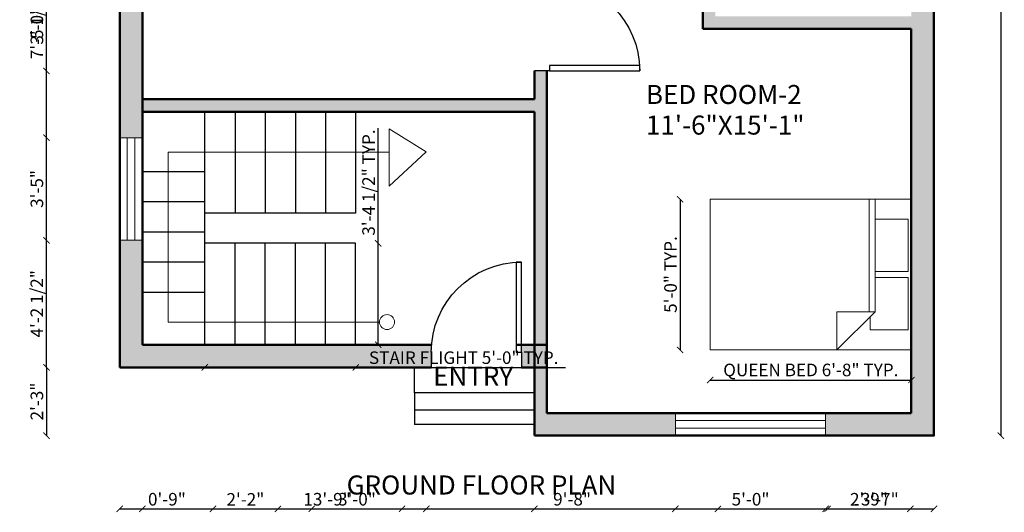
# Model space of a CAD drawing. Units: inches. Extents: x 1799 to 2247, y 1296 to 1881.
# Tile 1 of 4: x 1799 to 2190, y 1296 to 1492. Entities that reach past the tile are written whole.
import ezdxf

# ---------------------------------------------------------------- set-up
doc = ezdxf.new("R2010")
doc.units = ezdxf.units.IN
for name, color, linetype, lineweight in [('A-ANNO-DIMS', 2, 'Continuous', 18), ('A-ANNO-SYMB', 2, 'Continuous', 18), ('A-ANNO-TEXT', 7, 'Continuous', 35), ('A-AREA-IDEN', 7, 'Continuous', 25), ('A-DOOR', 3, 'Continuous', 25), ('A-FLOR-STRS', 7, 'Continuous', 25), ('A-FURN', 8, 'Continuous', 18), ('A-WALL', 7, 'Continuous', 50), ('window', 4, 'Continuous', 18)]:
    doc.layers.add(name, color=color, linetype=linetype, lineweight=lineweight)
doc.layers.add('A-WALL-PATT', color=18, linetype='Continuous', lineweight=13, true_color=0x000000)
doc.styles.get("Standard").update_dxf_attribs({"font": 'arial.ttf'})
doc.dimstyles.new('ISO-25', dxfattribs={"dimtxt": 5, "dimasz": 2.5, "dimexe": 1.25, "dimexo": 0.625, "dimtad": 1, "dimdec": 0, "dimlunit": 4, "dimtxsty": 'Standard', "dimblk": 'ARCHTICK', "dimcen": 2.5, "dimse1": 1, "dimse2": 1, "dimclrd": 1, "dimadec": 0, "dimazin": 0, "dimtfac": 1, "dimtdec": 0, "dimtmove": 0, "dimatfit": 3, "dimfxl": 1, "dimarcsym": 0})

# ---------------------------------------------------------------- blocks, each defined once
blk = doc.blocks.new('Bed - Queen')
for p, q in [((0, -80.00003), (0, 0)), ((0, 0), (59.99999, 0)), ((59.99999, 0), (59.99999, -80.00003)), ((7.99999, -1.2), (28.79998, -1.2)), ((7.99999, -14.4), (7.99999, -1.2)), ((28.79998, -1.2), (28.79998, -14.4)), ((31.19999, -1.2), (51.99999, -1.2)), ((31.19999, -14.4), (31.19999, -1.2)), ((51.99999, -1.2), (51.99999, -16.4)), ((0, -14.4), (44.8, -14.4)), ((59.99999, -29.6), (44.8, -14.4)), ((44.8, -14.4), (44.8, -29.6)), ((44.8, -16.8), (0, -16.8)), ((51.99999, -16.4), (46.79936, -16.4)), ((44.8, -29.6), (59.99999, -29.6)), ((59.99999, -80.00003), (0, -80.00003))]:
    blk.add_line(p, q)
blk = doc.blocks.new('*U12')
for p, q in [((0, 0), (0, -5)), ((30, 0), (30, -5))]:
    blk.add_line(p, q)
blk.add_lwpolyline([(0, 0), (0, 30), (1.75, 30), (1.75, 0)], close=True)
blk.add_arc((0, 0), 30, 0, 90)
blk = doc.blocks.new('_ArchTick')
at = {"color": 0, "linetype": 'ByBlock', "const_width": 0.15}
blk.add_lwpolyline([(-0.5, -0.5), (0.5, 0.5)], dxfattribs=at)
blk = doc.blocks.new('*D14')
at = {"layer": 'A-ANNO-DIMS', "color": 0, "lineweight": -2, "transparency": 16777216}
blk.add_line((2189.08, 1830.32), (2189.08, 1326.32), dxfattribs=at)
at = {"layer": 'Defpoints', "color": 0, "transparency": 16777216}
for p in [(2162.46, 1830.32), (2162.46, 1326.32), (2189.08, 1326.32)]:
    blk.add_point(p, dxfattribs=at)
at = {"layer": 'A-ANNO-DIMS', "color": 0, "lineweight": -2, "transparency": 16777216, "xscale": 2.5, "yscale": 2.5, "zscale": 2.5}
for p, rotation in [((2189.08, 1830.32), 90), ((2189.08, 1326.32), 270)]:
    blk.add_blockref('_ArchTick', p, dxfattribs=dict(at, rotation=rotation))
at = {"layer": 'A-ANNO-DIMS', "color": 0, "transparency": 16777216, "insert": (2185.95, 1578.32), "char_height": 5, "attachment_point": 5, "rotation": 90}
blk.add_mtext("42'", dxfattribs=at)
blk = doc.blocks.new('STAIR-FLIGHT-5-TREAD')
for p, q in [((60, 40.41), (0, 40.41)), ((12, 0), (12, 40.41)), ((24, 0), (24, 40.41)), ((36, 0), (36, 40.41)), ((48, 0), (48, 40.41)), ((60, 0), (60, 40.41))]:
    blk.add_line(p, q)
blk = doc.blocks.new('*D16')
at = {"layer": 'A-ANNO-DIMS', "color": 1, "lineweight": -2, "transparency": 16777216}
blk.add_line((2073.46, 1348.47), (2153.46, 1348.47), dxfattribs=at)
at = {"layer": 'Defpoints', "color": 0, "transparency": 16777216}
for p in [(2073.46, 1360.47), (2153.46, 1360.47), (2153.46, 1348.47)]:
    blk.add_point(p, dxfattribs=at)
at = {"layer": 'A-ANNO-DIMS', "color": 1, "lineweight": -2, "transparency": 16777216, "xscale": 2.5, "yscale": 2.5, "zscale": 2.5, "rotation": 180}
blk.add_blockref('_ArchTick', (2073.46, 1348.47), dxfattribs=at)
at = {"layer": 'A-ANNO-DIMS', "color": 1, "lineweight": -2, "transparency": 16777216, "xscale": 2.5, "yscale": 2.5, "zscale": 2.5}
blk.add_blockref('_ArchTick', (2153.46, 1348.47), dxfattribs=at)
at = {"layer": 'A-ANNO-DIMS', "color": 0, "transparency": 16777216, "insert": (2113.46, 1351.83), "char_height": 5, "attachment_point": 5}
blk.add_mtext('QUEEN BED 6\'-8" TYP.', dxfattribs=at)
blk = doc.blocks.new('*D17')
at = {"layer": 'A-ANNO-DIMS', "color": 1, "lineweight": -2, "transparency": 16777216}
blk.add_line((2061.46, 1420.47), (2061.46, 1360.47), dxfattribs=at)
at = {"layer": 'Defpoints', "color": 0, "transparency": 16777216}
for p in [(2073.46, 1420.47), (2061.46, 1360.47), (2073.46, 1360.47)]:
    blk.add_point(p, dxfattribs=at)
at = {"layer": 'A-ANNO-DIMS', "color": 1, "lineweight": -2, "transparency": 16777216, "xscale": 2.5, "yscale": 2.5, "zscale": 2.5}
for p, rotation in [((2061.46, 1420.47), 90), ((2061.46, 1360.47), 270)]:
    blk.add_blockref('_ArchTick', p, dxfattribs=dict(at, rotation=rotation))
at = {"layer": 'A-ANNO-DIMS', "color": 0, "transparency": 16777216, "insert": (2058.28, 1390.47), "char_height": 5, "attachment_point": 5, "rotation": 90}
blk.add_mtext('5\'-0" TYP.', dxfattribs=at)
blk = doc.blocks.new('*D20')
at = {"layer": 'A-ANNO-DIMS', "color": 1, "lineweight": -2, "transparency": 16777216}
for p, q in [((1872.34, 1353.51), (1932.34, 1353.51)), ((1932.34, 1353.51), (2015.83, 1353.51))]:
    blk.add_line(p, q, dxfattribs=at)
at = {"layer": 'Defpoints', "color": 0, "transparency": 16777216}
for p in [(1872.34, 1362.51), (1932.34, 1362.51), (1932.34, 1353.51)]:
    blk.add_point(p, dxfattribs=at)
at = {"layer": 'A-ANNO-DIMS', "color": 1, "lineweight": -2, "transparency": 16777216, "xscale": 2.5, "yscale": 2.5, "zscale": 2.5, "rotation": 180}
blk.add_blockref('_ArchTick', (1872.34, 1353.51), dxfattribs=at)
at = {"layer": 'A-ANNO-DIMS', "color": 1, "lineweight": -2, "transparency": 16777216, "xscale": 2.5, "yscale": 2.5, "zscale": 2.5}
blk.add_blockref('_ArchTick', (1932.34, 1353.51), dxfattribs=at)
at = {"layer": 'A-ANNO-DIMS', "color": 0, "transparency": 16777216, "insert": (1975.33, 1356.72), "char_height": 5, "attachment_point": 5}
blk.add_mtext('STAIR FLIGHT 5\'-0" TYP.', dxfattribs=at)
blk = doc.blocks.new('*D21')
at = {"layer": 'A-ANNO-DIMS', "color": 1, "lineweight": -2, "transparency": 16777216}
for p, q in [((1941.34, 1402.91), (1941.34, 1448.79)), ((1941.34, 1362.51), (1941.34, 1402.91))]:
    blk.add_line(p, q, dxfattribs=at)
at = {"layer": 'Defpoints', "color": 0, "transparency": 16777216}
for p in [(1932.34, 1402.91), (1941.34, 1402.91), (1932.34, 1362.51)]:
    blk.add_point(p, dxfattribs=at)
at = {"layer": 'A-ANNO-DIMS', "color": 1, "lineweight": -2, "transparency": 16777216, "xscale": 2.5, "yscale": 2.5, "zscale": 2.5}
for p, rotation in [((1941.34, 1402.91), 90), ((1941.34, 1362.51), 270)]:
    blk.add_blockref('_ArchTick', p, dxfattribs=dict(at, rotation=rotation))
at = {"layer": 'A-ANNO-DIMS', "color": 0, "transparency": 16777216, "insert": (1938.13, 1427.1), "char_height": 5, "attachment_point": 5, "rotation": 90}
blk.add_mtext('3\'-4 1/2" TYP.', dxfattribs=at)
blk = doc.blocks.new('*D32')
at = {"layer": 'A-ANNO-DIMS', "color": 1, "lineweight": -2, "transparency": 16777216}
blk.add_line((1838.46, 1297.17), (2003.46, 1297.17), dxfattribs=at)
at = {"layer": 'Defpoints', "color": 0, "transparency": 16777216}
for p in [(1838.46, 1353.51), (2003.46, 1326.32), (2003.46, 1297.17)]:
    blk.add_point(p, dxfattribs=at)
at = {"layer": 'A-ANNO-DIMS', "color": 1, "lineweight": -2, "transparency": 16777216, "xscale": 2.5, "yscale": 2.5, "zscale": 2.5, "rotation": 180}
blk.add_blockref('_ArchTick', (1838.46, 1297.17), dxfattribs=at)
at = {"layer": 'A-ANNO-DIMS', "color": 1, "lineweight": -2, "transparency": 16777216, "xscale": 2.5, "yscale": 2.5, "zscale": 2.5}
blk.add_blockref('_ArchTick', (2003.46, 1297.17), dxfattribs=at)
at = {"layer": 'A-ANNO-DIMS', "color": 0, "transparency": 16777216, "insert": (1920.96, 1300.35), "char_height": 5, "attachment_point": 5}
blk.add_mtext('13\'-9"', dxfattribs=at)
blk = doc.blocks.new('*D33')
at = {"layer": 'A-ANNO-DIMS', "color": 1, "lineweight": -2, "transparency": 16777216}
blk.add_line((1809.31, 1353.51), (1809.31, 1326.32), dxfattribs=at)
at = {"layer": 'Defpoints', "color": 0, "transparency": 16777216}
for p in [(1838.46, 1353.51), (1809.31, 1326.32), (2003.46, 1326.32)]:
    blk.add_point(p, dxfattribs=at)
at = {"layer": 'A-ANNO-DIMS', "color": 1, "lineweight": -2, "transparency": 16777216, "xscale": 2.5, "yscale": 2.5, "zscale": 2.5}
for p, rotation in [((1809.31, 1353.51), 90), ((1809.31, 1326.32), 270)]:
    blk.add_blockref('_ArchTick', p, dxfattribs=dict(at, rotation=rotation))
at = {"layer": 'A-ANNO-DIMS', "color": 0, "transparency": 16777216, "insert": (1806.13, 1339.91), "char_height": 5, "attachment_point": 5, "rotation": 90}
blk.add_mtext('2\'-3"', dxfattribs=at)
blk = doc.blocks.new('*D35')
at = {"layer": 'A-ANNO-DIMS', "color": 1, "lineweight": -2, "transparency": 16777216}
blk.add_line((1960.46, 1297.17), (2076.46, 1297.17), dxfattribs=at)
at = {"layer": 'Defpoints', "color": 0, "transparency": 16777216}
for p in [(1960.46, 1821.32), (2076.46, 1821.32), (2076.46, 1297.17)]:
    blk.add_point(p, dxfattribs=at)
at = {"layer": 'A-ANNO-DIMS', "color": 1, "lineweight": -2, "transparency": 16777216, "xscale": 2.5, "yscale": 2.5, "zscale": 2.5, "rotation": 180}
blk.add_blockref('_ArchTick', (1960.46, 1297.17), dxfattribs=at)
at = {"layer": 'A-ANNO-DIMS', "color": 1, "lineweight": -2, "transparency": 16777216, "xscale": 2.5, "yscale": 2.5, "zscale": 2.5}
blk.add_blockref('_ArchTick', (2076.46, 1297.17), dxfattribs=at)
at = {"layer": 'A-ANNO-DIMS', "color": 0, "transparency": 16777216, "insert": (2018.46, 1300.35), "char_height": 5, "attachment_point": 5}
blk.add_mtext('9\'-8"', dxfattribs=at)
blk = doc.blocks.new('*D37')
at = {"layer": 'A-ANNO-DIMS', "color": 1, "lineweight": -2, "transparency": 16777216}
blk.add_line((2119.37, 1297.17), (2162.46, 1297.17), dxfattribs=at)
at = {"layer": 'Defpoints', "color": 0, "transparency": 16777216}
for p in [(2119.37, 1326.32), (2162.46, 1326.32), (2162.46, 1297.17)]:
    blk.add_point(p, dxfattribs=at)
at = {"layer": 'A-ANNO-DIMS', "color": 1, "lineweight": -2, "transparency": 16777216, "xscale": 2.5, "yscale": 2.5, "zscale": 2.5, "rotation": 180}
blk.add_blockref('_ArchTick', (2119.37, 1297.17), dxfattribs=at)
at = {"layer": 'A-ANNO-DIMS', "color": 1, "lineweight": -2, "transparency": 16777216, "xscale": 2.5, "yscale": 2.5, "zscale": 2.5}
blk.add_blockref('_ArchTick', (2162.46, 1297.17), dxfattribs=at)
at = {"layer": 'A-ANNO-DIMS', "color": 0, "transparency": 16777216, "insert": (2140.92, 1300.35), "char_height": 5, "attachment_point": 5}
blk.add_mtext('3\'-7"', dxfattribs=at)
blk = doc.blocks.new('*D38')
at = {"layer": 'A-ANNO-DIMS', "color": 1, "lineweight": -2, "transparency": 16777216}
blk.add_line((2059.58, 1297.17), (2119.37, 1297.17), dxfattribs=at)
at = {"layer": 'Defpoints', "color": 0, "transparency": 16777216}
for p in [(2059.58, 1326.32), (2119.37, 1326.32), (2119.37, 1297.17)]:
    blk.add_point(p, dxfattribs=at)
at = {"layer": 'A-ANNO-DIMS', "color": 1, "lineweight": -2, "transparency": 16777216, "xscale": 2.5, "yscale": 2.5, "zscale": 2.5, "rotation": 180}
blk.add_blockref('_ArchTick', (2059.58, 1297.17), dxfattribs=at)
at = {"layer": 'A-ANNO-DIMS', "color": 1, "lineweight": -2, "transparency": 16777216, "xscale": 2.5, "yscale": 2.5, "zscale": 2.5}
blk.add_blockref('_ArchTick', (2119.37, 1297.17), dxfattribs=at)
at = {"layer": 'A-ANNO-DIMS', "color": 0, "transparency": 16777216, "insert": (2089.48, 1300.35), "char_height": 5, "attachment_point": 5}
blk.add_mtext('5\'-0"', dxfattribs=at)
blk = doc.blocks.new('*D47')
at = {"layer": 'A-ANNO-DIMS', "color": 1, "lineweight": -2, "transparency": 16777216}
blk.add_line((1914.89, 1297.17), (1950.83, 1297.17), dxfattribs=at)
at = {"layer": 'Defpoints', "color": 0, "transparency": 16777216}
for p in [(1914.89, 1701.32), (1950.83, 1701.32), (1950.83, 1297.17)]:
    blk.add_point(p, dxfattribs=at)
at = {"layer": 'A-ANNO-DIMS', "color": 1, "lineweight": -2, "transparency": 16777216, "xscale": 2.5, "yscale": 2.5, "zscale": 2.5, "rotation": 180}
blk.add_blockref('_ArchTick', (1914.89, 1297.17), dxfattribs=at)
at = {"layer": 'A-ANNO-DIMS', "color": 1, "lineweight": -2, "transparency": 16777216, "xscale": 2.5, "yscale": 2.5, "zscale": 2.5}
blk.add_blockref('_ArchTick', (1950.83, 1297.17), dxfattribs=at)
at = {"layer": 'A-ANNO-DIMS', "color": 0, "transparency": 16777216, "insert": (1932.86, 1300.35), "char_height": 5, "attachment_point": 5}
blk.add_mtext('3\'-0"', dxfattribs=at)
blk = doc.blocks.new('*D48')
at = {"layer": 'A-ANNO-DIMS', "color": 1, "lineweight": -2, "transparency": 16777216}
blk.add_line((1962.42, 1859.47), (1998.36, 1859.47), dxfattribs=at)
at = {"layer": 'Defpoints', "color": 0, "transparency": 16777216}
for p in [(1998.36, 1859.47), (1962.42, 1353.51), (1998.36, 1353.51)]:
    blk.add_point(p, dxfattribs=at)
at = {"layer": 'A-ANNO-DIMS', "color": 1, "lineweight": -2, "transparency": 16777216, "xscale": 2.5, "yscale": 2.5, "zscale": 2.5, "rotation": 180}
blk.add_blockref('_ArchTick', (1962.42, 1859.47), dxfattribs=at)
at = {"layer": 'A-ANNO-DIMS', "color": 1, "lineweight": -2, "transparency": 16777216, "xscale": 2.5, "yscale": 2.5, "zscale": 2.5}
blk.add_blockref('_ArchTick', (1998.36, 1859.47), dxfattribs=at)
at = {"layer": 'A-ANNO-DIMS', "color": 0, "transparency": 16777216, "insert": (1980.39, 1862.65), "char_height": 5, "attachment_point": 5}
blk.add_mtext('3\'-0"', dxfattribs=at)
blk = doc.blocks.new('*D50')
at = {"layer": 'A-ANNO-DIMS', "color": 1, "lineweight": -2, "transparency": 16777216}
blk.add_line((1809.31, 1444.97), (1809.31, 1534.31), dxfattribs=at)
at = {"layer": 'Defpoints', "color": 0, "transparency": 16777216}
for p in [(1809.31, 1534.31), (1838.46, 1534.31), (1838.46, 1444.97)]:
    blk.add_point(p, dxfattribs=at)
at = {"layer": 'A-ANNO-DIMS', "color": 1, "lineweight": -2, "transparency": 16777216, "xscale": 2.5, "yscale": 2.5, "zscale": 2.5}
for p, rotation in [((1809.31, 1534.31), 90), ((1809.31, 1444.97), 270)]:
    blk.add_blockref('_ArchTick', p, dxfattribs=dict(at, rotation=rotation))
at = {"layer": 'A-ANNO-DIMS', "color": 0, "transparency": 16777216, "insert": (1806.1, 1489.64), "char_height": 5, "attachment_point": 5, "rotation": 90}
blk.add_mtext('7\'-5 1/2"', dxfattribs=at)
blk = doc.blocks.new('*D51')
at = {"layer": 'A-ANNO-DIMS', "color": 1, "lineweight": -2, "transparency": 16777216}
blk.add_line((1809.31, 1404.13), (1809.31, 1444.97), dxfattribs=at)
at = {"layer": 'Defpoints', "color": 0, "transparency": 16777216}
for p in [(1809.31, 1444.97), (1838.46, 1444.97), (1838.46, 1404.13)]:
    blk.add_point(p, dxfattribs=at)
at = {"layer": 'A-ANNO-DIMS', "color": 1, "lineweight": -2, "transparency": 16777216, "xscale": 2.5, "yscale": 2.5, "zscale": 2.5}
for p, rotation in [((1809.31, 1444.97), 90), ((1809.31, 1404.13), 270)]:
    blk.add_blockref('_ArchTick', p, dxfattribs=dict(at, rotation=rotation))
at = {"layer": 'A-ANNO-DIMS', "color": 0, "transparency": 16777216, "insert": (1806.13, 1424.55), "char_height": 5, "attachment_point": 5, "rotation": 90}
blk.add_mtext('3\'-5"', dxfattribs=at)
blk = doc.blocks.new('*D52')
at = {"layer": 'A-ANNO-DIMS', "color": 1, "lineweight": -2, "transparency": 16777216}
blk.add_line((1809.31, 1353.51), (1809.31, 1404.13), dxfattribs=at)
at = {"layer": 'Defpoints', "color": 0, "transparency": 16777216}
for p in [(1809.31, 1404.13), (1838.46, 1404.13), (1838.46, 1353.51)]:
    blk.add_point(p, dxfattribs=at)
at = {"layer": 'A-ANNO-DIMS', "color": 1, "lineweight": -2, "transparency": 16777216, "xscale": 2.5, "yscale": 2.5, "zscale": 2.5}
for p, rotation in [((1809.31, 1404.13), 90), ((1809.31, 1353.51), 270)]:
    blk.add_blockref('_ArchTick', p, dxfattribs=dict(at, rotation=rotation))
at = {"layer": 'A-ANNO-DIMS', "color": 0, "transparency": 16777216, "insert": (1806.1, 1378.82), "char_height": 5, "attachment_point": 5, "rotation": 90}
blk.add_mtext('4\'-2 1/2"', dxfattribs=at)
blk = doc.blocks.new('*D57')
at = {"layer": 'A-ANNO-DIMS', "color": 1, "lineweight": -2, "transparency": 16777216}
blk.add_line((1875.53, 1297.17), (1901.39, 1297.17), dxfattribs=at)
at = {"layer": 'Defpoints', "color": 0, "transparency": 16777216}
for p in [(1901.39, 1801.76), (1875.53, 1797.03), (1901.39, 1297.17)]:
    blk.add_point(p, dxfattribs=at)
at = {"layer": 'A-ANNO-DIMS', "color": 1, "lineweight": -2, "transparency": 16777216, "xscale": 2.5, "yscale": 2.5, "zscale": 2.5, "rotation": 180}
blk.add_blockref('_ArchTick', (1875.53, 1297.17), dxfattribs=at)
at = {"layer": 'A-ANNO-DIMS', "color": 1, "lineweight": -2, "transparency": 16777216, "xscale": 2.5, "yscale": 2.5, "zscale": 2.5}
blk.add_blockref('_ArchTick', (1901.39, 1297.17), dxfattribs=at)
at = {"layer": 'A-ANNO-DIMS', "color": 0, "transparency": 16777216, "insert": (1888.46, 1300.3), "char_height": 5, "attachment_point": 5}
blk.add_mtext('2\'-2"', dxfattribs=at)
blk = doc.blocks.new('*D60')
at = {"layer": 'A-ANNO-DIMS', "color": 1, "lineweight": -2, "transparency": 16777216}
blk.add_line((1809.31, 1471.58), (1809.31, 1507.52), dxfattribs=at)
at = {"layer": 'Defpoints', "color": 0, "transparency": 16777216}
for p in [(1809.31, 1507.52), (2003.46, 1507.52), (2003.46, 1471.58)]:
    blk.add_point(p, dxfattribs=at)
at = {"layer": 'A-ANNO-DIMS', "color": 1, "lineweight": -2, "transparency": 16777216, "xscale": 2.5, "yscale": 2.5, "zscale": 2.5}
for p, rotation in [((1809.31, 1507.52), 90), ((1809.31, 1471.58), 270)]:
    blk.add_blockref('_ArchTick', p, dxfattribs=dict(at, rotation=rotation))
at = {"layer": 'A-ANNO-DIMS', "color": 0, "transparency": 16777216, "insert": (1806.13, 1489.55), "char_height": 5, "attachment_point": 5, "rotation": 90}
blk.add_mtext('3\'-0"', dxfattribs=at)
blk = doc.blocks.new('*D61')
at = {"layer": 'A-ANNO-DIMS', "color": 1, "lineweight": -2, "transparency": 16777216}
for p, q in [((1838.46, 1297.17), (1847.46, 1297.17)), ((1847.46, 1297.17), (1864.5, 1297.17))]:
    blk.add_line(p, q, dxfattribs=at)
at = {"layer": 'Defpoints', "color": 0, "transparency": 16777216}
for p in [(1838.46, 1830.32), (1847.46, 1821.32), (1847.46, 1297.17)]:
    blk.add_point(p, dxfattribs=at)
at = {"layer": 'A-ANNO-DIMS', "color": 1, "lineweight": -2, "transparency": 16777216, "xscale": 2.5, "yscale": 2.5, "zscale": 2.5, "rotation": 180}
blk.add_blockref('_ArchTick', (1838.46, 1297.17), dxfattribs=at)
at = {"layer": 'A-ANNO-DIMS', "color": 1, "lineweight": -2, "transparency": 16777216, "xscale": 2.5, "yscale": 2.5, "zscale": 2.5}
blk.add_blockref('_ArchTick', (1847.46, 1297.17), dxfattribs=at)
at = {"layer": 'A-ANNO-DIMS', "color": 0, "transparency": 16777216, "insert": (1857.23, 1300.35), "char_height": 5, "attachment_point": 5}
blk.add_mtext('0\'-9"', dxfattribs=at)
blk = doc.blocks.new('*D66')
at = {"layer": 'A-ANNO-DIMS', "color": 1, "lineweight": -2, "transparency": 16777216}
blk.add_line((2120.1, 1297.17), (2153.1, 1297.17), dxfattribs=at)
at = {"layer": 'Defpoints', "color": 0, "transparency": 16777216}
for p in [(2120.1, 1525.25), (2153.1, 1514.75), (2153.1, 1297.17)]:
    blk.add_point(p, dxfattribs=at)
at = {"layer": 'A-ANNO-DIMS', "color": 1, "lineweight": -2, "transparency": 16777216, "xscale": 2.5, "yscale": 2.5, "zscale": 2.5, "rotation": 180}
blk.add_blockref('_ArchTick', (2120.1, 1297.17), dxfattribs=at)
at = {"layer": 'A-ANNO-DIMS', "color": 1, "lineweight": -2, "transparency": 16777216, "xscale": 2.5, "yscale": 2.5, "zscale": 2.5}
blk.add_blockref('_ArchTick', (2153.1, 1297.17), dxfattribs=at)
at = {"layer": 'A-ANNO-DIMS', "color": 0, "transparency": 16777216, "insert": (2136.6, 1300.35), "char_height": 5, "attachment_point": 5}
blk.add_mtext('2\'-9"', dxfattribs=at)

msp = doc.modelspace()

# ---------------------------------------------------------------- hatches: boundary and pattern name
at = {"layer": 'A-WALL-PATT'}
h = msp.add_hatch(color=256, dxfattribs=at)
h.dxf.hatch_style = 1
h.paths.add_polyline_path([(1847.46, 1821.32), (1883.11, 1821.32), (1883.11, 1830.32), (1838.46, 1830.32), (1838.46, 1618.8), (1847.46, 1618.8)])
h.paths.add_polyline_path([(1847.46, 1534.31), (1838.46, 1534.31), (1838.46, 1444.97), (1847.46, 1444.97)])
h.paths.add_polyline_path([(1847.46, 1404.13), (1838.46, 1404.13), (1838.46, 1353.51), (1847.46, 1353.51), (1962.42, 1353.51), (1962.42, 1359.5, -0.020971), (1962.55, 1362.51), (1847.46, 1362.51)])
h.paths.add_polyline_path([(2162.46, 1509.73), (2153.46, 1509.73), (2153.46, 1493.32), (2075.46, 1493.32), (2075.46, 1496.56), (2075.02, 1496.56), (2070.46, 1496.56), (2070.46, 1488.32), (2153.46, 1488.32), (2153.46, 1335.32), (2119.37, 1335.32), (2119.37, 1326.32), (2162.46, 1326.32)])
h.paths.add_polyline_path([(2059.58, 1335.32), (2008.46, 1335.32), (2008.46, 1353.51), (2003.46, 1353.51), (2003.46, 1335.32), (2003.46, 1326.32), (2059.58, 1326.32)])
h.paths.add_polyline_path([(2008.46, 1471.58), (2003.46, 1471.58), (2003.46, 1460.32), (1847.46, 1460.32), (1847.46, 1455.32), (2003.46, 1455.32), (2003.46, 1362.51), (2008.46, 1362.51)])
h.paths.add_polyline_path([(2008.46, 1362.51), (2003.46, 1362.51), (2003.46, 1353.51), (2008.46, 1353.51)])
h.paths.add_polyline_path([(2003.46, 1362.51), (1998.36, 1362.51), (1998.36, 1359.5), (1998.36, 1353.51), (2003.46, 1353.51)])
h.paths.add_polyline_path([(1989.49, 1830.32), (1953.2, 1830.32), (1953.2, 1821.32), (1955.46, 1821.32), (1955.46, 1701.32), (1950.83, 1701.32), (1950.83, 1696.32), (1960.46, 1696.32), (1960.46, 1821.32), (1989.49, 1821.32)])
h.paths.add_polyline_path([(2162.46, 1606.83), (2153.46, 1606.83), (2153.46, 1541.93), (2162.46, 1541.93)])
h.paths.add_polyline_path([(2162.46, 1746.71), (2153.46, 1746.71), (2153.46, 1701.32), (2081.46, 1701.32), (2081.46, 1707.91), (2081.05, 1707.91), (2076.46, 1707.91), (2076.46, 1701.32), (2003.46, 1701.32), (2003.46, 1604.81), (2008.46, 1604.81), (2008.46, 1696.32), (2153.46, 1696.32), (2153.46, 1656.83), (2162.46, 1656.83)])
h.paths.add_polyline_path([(2162.46, 1830.32), (2050.89, 1830.32), (2050.89, 1821.32), (2076.46, 1821.32), (2076.46, 1735.44), (2081.05, 1735.44, -0.003736), (2081.46, 1735.44), (2081.46, 1821.32), (2153.46, 1821.32), (2153.46, 1778.8), (2162.46, 1778.8)])
h.paths.add_polyline_path([(1961.29, 1344.27), (2000.99, 1344.27), (2000.99, 1355.65), (1961.29, 1355.65)], flags=9)
h.paths.add_polyline_path([(1882.83, 1491.06), (1947.74, 1491.06), (1947.74, 1502.69), (1882.83, 1502.69)], flags=9)
h.paths.add_polyline_path([(1882.8, 1503.23), (1950.9, 1503.23), (1950.9, 1514.99), (1882.8, 1514.99)], flags=9)
h.paths.add_polyline_path([(2045.91, 1444.14), (2110.82, 1444.14), (2110.82, 1455.75), (2045.91, 1455.75)], flags=9)
h.paths.add_polyline_path([(2045.88, 1456.29), (2116.91, 1456.29), (2116.91, 1468.06), (2045.88, 1468.06)], flags=9)
h.paths.add_polyline_path([(2084.43, 1526.38), (2124.38, 1526.38), (2124.38, 1537.99), (2084.43, 1537.99)], flags=9)
h.paths.add_polyline_path([(2084.4, 1538.53), (2125.41, 1538.53), (2125.41, 1550.3), (2084.4, 1550.3)], flags=9)
h.paths.add_polyline_path([(2013.59, 1530.05), (2066.72, 1530.05), (2066.72, 1541.67), (2013.59, 1541.67)], flags=9)
h.paths.add_polyline_path([(2013.56, 1542.21), (2053.98, 1542.21), (2053.98, 1553.97), (2013.56, 1553.97)], flags=9)
h.paths.add_polyline_path([(2054.17, 1583.99), (2119.08, 1583.99), (2119.08, 1595.62), (2054.17, 1595.62)], flags=9)
h.paths.add_polyline_path([(2054.14, 1596.16), (2125.17, 1596.16), (2125.17, 1607.93), (2054.14, 1607.93)], flags=9)
h.paths.add_polyline_path([(2091.32, 1783.78), (2144.45, 1783.78), (2144.45, 1795.39), (2091.32, 1795.39)], flags=25)
h.paths.add_polyline_path([(2091.3, 1795.93), (2142.9, 1795.93), (2142.9, 1807.7), (2091.3, 1807.7)], flags=25)
h.paths.add_polyline_path([(1985.13, 1779.5), (2017.8, 1779.5), (2017.8, 1790.88), (1985.13, 1790.88)], flags=9)
h.paths.add_polyline_path([(1985.08, 1791.49), (2020.79, 1791.49), (2020.79, 1803.25), (1985.08, 1803.25)], flags=9)
h.paths.add_polyline_path([(1879.15, 1761.55), (1938.17, 1761.55), (1938.17, 1773.17), (1879.15, 1773.17)], flags=9)
h.paths.add_polyline_path([(1879.13, 1773.71), (1929.55, 1773.71), (1929.55, 1785.47), (1879.13, 1785.47)], flags=9)

# ---------------------------------------------------------------- linework, layer by layer
at = {"layer": 'A-ANNO-SYMB'}
for p, q in [((1945.62, 1439.15), (1945.62, 1448.48)), ((1945.62, 1448.48), (1960.37, 1439.27)), ((1857.67, 1371.55), (1857.67, 1439.15)), ((1857.67, 1439.15), (1945.62, 1439.15)), ((1960.37, 1439.27), (1945.62, 1425.67)), ((1945.62, 1425.67), (1945.62, 1439.15)), ((1941.83, 1371.55), (1857.67, 1371.55))]:
    msp.add_line(p, q, dxfattribs=at)
msp.add_circle((1944.82, 1371.55), 2.99, dxfattribs=at)
at = {"layer": 'A-FLOR-STRS'}
for p, q in [((1872.34, 1362.51), (1872.34, 1455.32)), ((1872.34, 1431.38), (1847.46, 1431.38)), ((1872.34, 1419.38), (1847.46, 1419.38)), ((1872.34, 1407.38), (1847.46, 1407.38)), ((1872.34, 1395.38), (1847.46, 1395.38)), ((1872.34, 1383.38), (1847.46, 1383.38)), ((1955.8, 1343.4), (1955.8, 1353.51)), ((2003.46, 1343.4), (1955.8, 1343.4)), ((1955.8, 1343.4), (1955.8, 1330.82)), ((2003.46, 1336.5), (1955.8, 1336.5)), ((2003.46, 1330.82), (1955.8, 1330.82))]:
    msp.add_line(p, q, dxfattribs=at)
at = {"layer": 'A-WALL'}
for p, q in [((1847.46, 1362.51), (1847.46, 1821.32)), ((2070.46, 1496.56), (2070.46, 1488.32)), ((2070.46, 1488.32), (2153.46, 1488.32)), ((2153.46, 1488.32), (2153.46, 1335.32)), ((2003.46, 1460.32), (2003.46, 1471.58)), ((2008.46, 1335.32), (2008.46, 1471.58)), ((1847.46, 1460.32), (2003.46, 1460.32)), ((1847.46, 1455.32), (2003.46, 1455.32)), ((2003.46, 1335.32), (2003.46, 1455.32)), ((1847.46, 1362.51), (1962.55, 1362.51)), ((1996.26, 1362.51), (2008.46, 1362.51)), ((1847.46, 1353.51), (1838.46, 1353.51)), ((1847.46, 1353.51), (1962.42, 1353.51)), ((1998.36, 1353.51), (2008.46, 1353.51)), ((2003.46, 1335.32), (2003.46, 1326.32)), ((2153.46, 1335.32), (2008.46, 1335.32))]:
    msp.add_line(p, q, dxfattribs=at)
msp.add_lwpolyline([(1838.46, 1353.51), (1838.46, 1830.32), (2162.46, 1830.32), (2162.46, 1326.32), (2003.46, 1326.32)], dxfattribs=at)
at = {"layer": 'window'}
for p, q in [((1847.46, 1444.97), (1838.46, 1444.97)), ((1838.46, 1444.97), (1838.46, 1404.13)), ((1841.46, 1444.97), (1841.46, 1404.13)), ((1844.46, 1444.97), (1844.46, 1404.13)), ((1847.46, 1404.13), (1847.46, 1444.97)), ((1838.46, 1404.13), (1847.46, 1404.13)), ((2059.58, 1335.32), (2059.58, 1326.32)), ((2119.37, 1335.32), (2059.58, 1335.32)), ((2059.58, 1332.32), (2119.37, 1332.32)), ((2119.37, 1326.32), (2119.37, 1335.32)), ((2059.58, 1329.32), (2119.37, 1329.32)), ((2059.58, 1326.32), (2119.37, 1326.32))]:
    msp.add_line(p, q, dxfattribs=at)

# ---------------------------------------------------------------- block references
at = {"layer": 'A-DOOR', "xscale": -1.197883670562129, "yscale": 1.197883670562129, "zscale": 1.197883670562129, "rotation": 270}
msp.add_blockref('*U12', (2009.45, 1471.58), dxfattribs=at)
at = {"layer": 'A-DOOR', "xscale": -1.197883670562129, "yscale": 1.197883670562129, "zscale": 1.197883670562129}
msp.add_blockref('*U12', (1998.36, 1359.5), dxfattribs=at)
at = {"layer": 'A-FLOR-STRS', "extrusion": (0, 0, -1), "zscale": -1, "rotation": 180}
msp.add_blockref('STAIR-FLIGHT-5-TREAD', (-1872.34, 1455.32), dxfattribs=at)
at = {"layer": 'A-FLOR-STRS'}
msp.add_blockref('STAIR-FLIGHT-5-TREAD', (1872.34, 1362.51), dxfattribs=at)
at = {"layer": 'A-FURN', "rotation": 270}
msp.add_blockref('Bed - Queen', (2153.46, 1420.47), dxfattribs=at)

# ---------------------------------------------------------------- texts
at = {"layer": 'A-ANNO-TEXT'}
msp.add_text('GROUND FLOOR PLAN', height=7.5834, dxfattribs=at).set_placement((1928.74, 1302.88))
at = {"layer": 'A-AREA-IDEN'}
for s, height, p in [('BED ROOM-2', 7.583, (2047.85, 1458.38)), ('11\'-6"X15\'-1"', 7.5834, (2047.85, 1446.2)), ('ENTRY', 7.583, (1963.19, 1346.17))]:
    msp.add_text(s, height=height, dxfattribs=at).set_placement(p)

# ---------------------------------------------------------------- dimensions: what is measured, and where the dimension line sits
at = {"layer": 'A-ANNO-DIMS'}
for base, p1, p2, picture, middle in [((1998.36, 1859.47), (1962.42, 1353.51), (1998.36, 1353.51), '*D48', (1980.39, 1862.65)), ((1847.46, 1297.17), (1838.46, 1830.32), (1847.46, 1821.32), '*D61', (1857.23, 1300.35)), ((2076.46, 1297.17), (1960.46, 1821.32), (2076.46, 1821.32), '*D35', (2018.46, 1300.35)), ((1901.39, 1297.17), (1875.53, 1797.03), (1901.39, 1801.76), '*D57', (1888.46, 1300.3)), ((1950.83, 1297.17), (1914.89, 1701.32), (1950.83, 1701.32), '*D47', (1932.86, 1300.35)), ((2153.1, 1297.17), (2120.1, 1525.25), (2153.1, 1514.75), '*D66', (2136.6, 1300.35)), ((2003.46, 1297.17), (1838.46, 1353.51), (2003.46, 1326.32), '*D32', (1920.96, 1300.35)), ((2119.37, 1297.17), (2059.58, 1326.32), (2119.37, 1326.32), '*D38', (2089.48, 1300.35)), ((2162.46, 1297.17), (2119.37, 1326.32), (2162.46, 1326.32), '*D37', (2140.92, 1300.35))]:
    dim = msp.add_linear_dim(base=base, p1=p1, p2=p2, dimstyle='ISO-25', override={"dimdec": 1, "dimlfac": 1, "dimrnd": 0, "dimzin": 1, "dimdsep": 46, "dimlunit": 4, "dimfrac": 2}, dxfattribs=at)
    dim.commit()
    dim.dimension.update_dxf_attribs({"geometry": picture, "text_midpoint": middle})
for base, p1, p2, override, picture, middle in [((2189.08, 1326.32), (2162.46, 1830.32), (2162.46, 1326.32), {"dimclrd": 0, "dimclre": 0, "dimclrt": 0}, '*D14', (2185.95, 1578.32)), ((1809.31, 1534.31), (1838.46, 1444.97), (1838.46, 1534.31), {"dimdec": 1, "dimlfac": 1, "dimrnd": 0, "dimzin": 1, "dimdsep": 46, "dimlunit": 4, "dimfrac": 2}, '*D50', (1806.1, 1489.64)), ((1809.31, 1507.52), (2003.46, 1471.58), (2003.46, 1507.52), {"dimdec": 1, "dimlfac": 1, "dimrnd": 0, "dimzin": 1, "dimdsep": 46, "dimlunit": 4, "dimfrac": 2}, '*D60', (1806.13, 1489.55)), ((1809.31, 1444.97), (1838.46, 1404.13), (1838.46, 1444.97), {"dimdec": 1, "dimlfac": 1, "dimrnd": 0, "dimzin": 1, "dimdsep": 46, "dimlunit": 4, "dimfrac": 2}, '*D51', (1806.13, 1424.55)), ((1809.31, 1404.13), (1838.46, 1353.51), (1838.46, 1404.13), {"dimdec": 1, "dimlfac": 1, "dimrnd": 0, "dimzin": 1, "dimdsep": 46, "dimlunit": 4, "dimfrac": 2}, '*D52', (1806.1, 1378.82)), ((1809.31, 1326.32), (1838.46, 1353.51), (2003.46, 1326.32), {"dimdec": 1, "dimlfac": 1, "dimrnd": 0, "dimzin": 1, "dimdsep": 46, "dimlunit": 4, "dimfrac": 2}, '*D33', (1806.13, 1339.91))]:
    dim = msp.add_linear_dim(base=base, p1=p1, p2=p2, angle=90, dimstyle='ISO-25', override=override, dxfattribs=at)
    dim.commit()
    dim.dimension.update_dxf_attribs({"geometry": picture, "text_midpoint": middle})
for base, p1, p2, angle, picture, middle in [((1941.34, 1402.91), (1932.34, 1362.51), (1932.34, 1402.91), 90, '*D21', (1938.13, 1427.1)), ((2061.46, 1360.47), (2073.46, 1420.47), (2073.46, 1360.47), 270, '*D17', (2058.28, 1390.47))]:
    dim = msp.add_linear_dim(base=base, p1=p1, p2=p2, angle=angle, text='<> TYP.', dimstyle='ISO-25', override={"dimdec": 1, "dimlfac": 1, "dimrnd": 0, "dimzin": 1, "dimdsep": 46, "dimlunit": 4, "dimfrac": 2}, dxfattribs=at)
    dim.commit()
    dim.dimension.update_dxf_attribs({"geometry": picture, "text_midpoint": middle})
for base, p1, p2, text, picture, middle in [((1932.34, 1353.51), (1872.34, 1362.51), (1932.34, 1362.51), 'STAIR FLIGHT <> TYP.', '*D20', (1975.33, 1356.72)), ((2153.46, 1348.47), (2073.46, 1360.47), (2153.46, 1360.47), 'QUEEN BED <> TYP.', '*D16', (2113.46, 1351.83))]:
    dim = msp.add_linear_dim(base=base, p1=p1, p2=p2, text=text, dimstyle='ISO-25', override={"dimdec": 1, "dimlfac": 1, "dimrnd": 0, "dimzin": 1, "dimdsep": 46, "dimlunit": 4, "dimfrac": 2}, dxfattribs=at)
    dim.commit()
    dim.dimension.update_dxf_attribs({"geometry": picture, "text_midpoint": middle})

doc.saveas('drawing.dxf')
